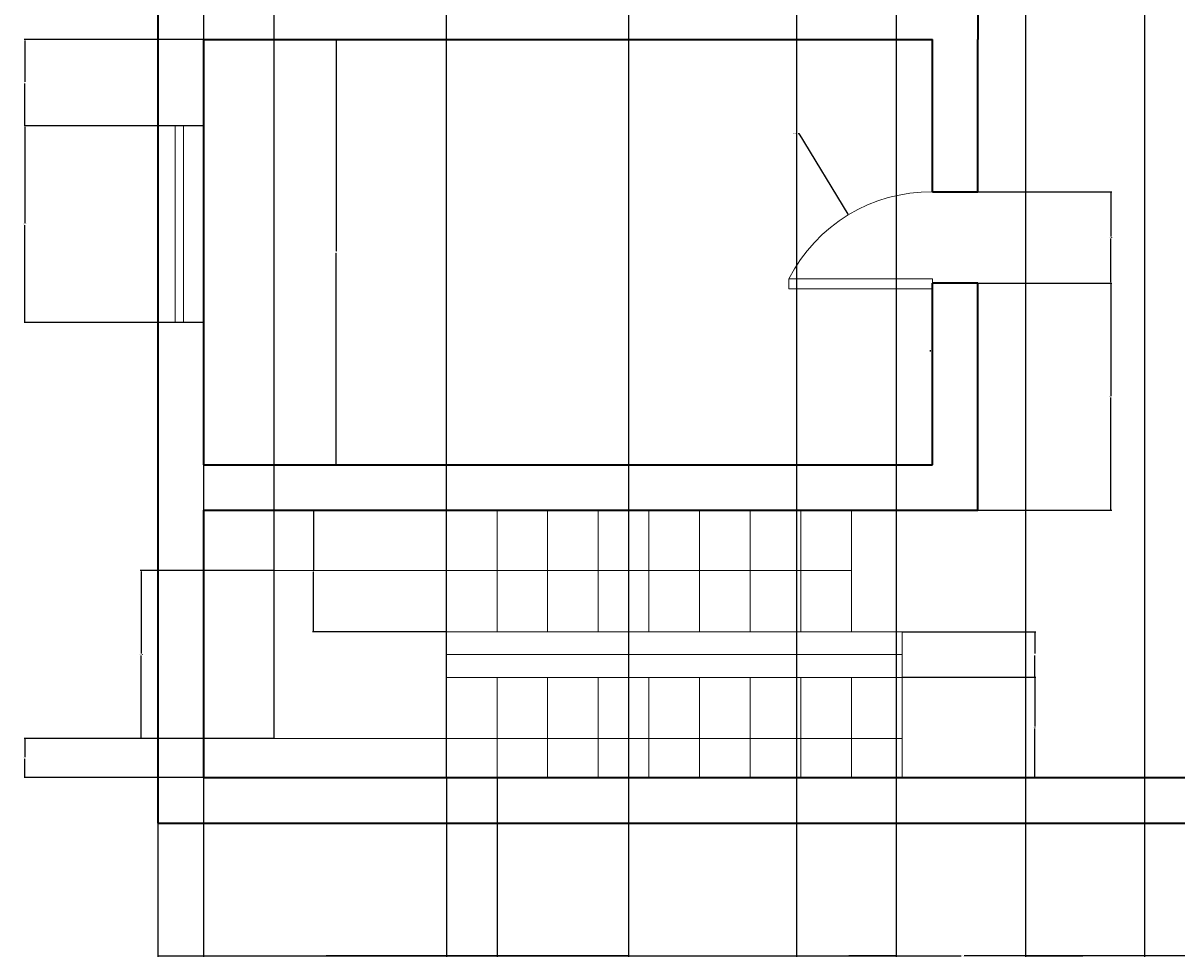
# Model space of a CAD drawing. Units: inches. Extents: x -20 to 351, y -512 to 63.
# Tile 1 of 5: x -20 to 208, y -512 to -328. Entities that reach past the tile are written whole.
import ezdxf

# ---------------------------------------------------------------- set-up
doc = ezdxf.new("R2010")
doc.units = ezdxf.units.IN
doc.header["$MEASUREMENT"] = 0
for name, color, linetype, lineweight in [('A-ANNO-DIMS', 2, 'Continuous', 18), ('A-DOOR', 3, 'Continuous', 18), ('A-FLOR-STRS', 7, 'Continuous', 18), ('A-GLAZ', 4, 'Continuous', 18), ('A-WALL', 7, 'Continuous', 35)]:
    doc.layers.add(name, color=color, linetype=linetype, lineweight=lineweight)
doc.styles.get("Standard").update_dxf_attribs({"font": 'arial.ttf'})
doc.dimstyles.get("Standard").update_dxf_attribs({"dimtxt": 0.18, "dimasz": 0.18, "dimexe": 0.18, "dimexo": 0.0625, "dimgap": 0.09, "dimtad": 0, "dimtih": 1, "dimtoh": 1, "dimdec": 4, "dimzin": 0, "dimdsep": 46, "dimtxsty": 'Standard', "dimcen": 0.09, "dimadec": 0, "dimazin": 0, "dimtfac": 1, "dimtdec": 4, "dimtofl": 0, "dimtmove": 0, "dimatfit": 3, "dimfxl": 1, "dimtolj": 1, "dimtzin": 0, "dimarcsym": 0})

# ---------------------------------------------------------------- blocks, each defined once
blk = doc.blocks.new('*D9')
at = {"layer": 'A-ANNO-DIMS', "color": 0, "lineweight": -2, "transparency": 16777216}
for p, q in [((324.28, -315.88), (324.28, -512.19)), ((6.28, -485.83), (6.28, -512.19)), ((6.46, -512.01), (165, -512.01)), ((324.1, -512.01), (165.57, -512.01))]:
    blk.add_line(p, q, dxfattribs=at)
at = {"layer": 'A-ANNO-DIMS', "color": 0, "transparency": 16777216}
for points in [[(6.46, -511.98), (6.46, -512.04), (6.28, -512.01)], [(324.1, -511.98), (324.1, -512.04), (324.28, -512.01)]]:
    blk.add_solid(points, dxfattribs=at)
at = {"layer": 'Defpoints', "color": 0, "transparency": 16777216}
for p in [(324.28, -315.82), (6.28, -485.76), (324.28, -512.01)]:
    blk.add_point(p, dxfattribs=at)
at = {"layer": 'A-ANNO-DIMS', "color": 0, "transparency": 16777216, "insert": (165.28, -512.01), "char_height": 0.18, "attachment_point": 5}
blk.add_mtext('\\A1;318', dxfattribs=at)
blk = doc.blocks.new('*D20')
at = {"layer": 'A-ANNO-DIMS', "color": 0, "lineweight": -2, "transparency": 16777216}
for p, q in [((15.22, -330.96), (-20.15, -330.96)), ((-19.97, -331.14), (-19.97, -339.31)), ((-19.97, -347.84), (-19.97, -339.67)), ((15.22, -348.02), (-20.15, -348.02))]:
    blk.add_line(p, q, dxfattribs=at)
at = {"layer": 'A-ANNO-DIMS', "color": 0, "transparency": 16777216}
for points in [[(-20, -331.14), (-19.94, -331.14), (-19.97, -330.96)], [(-20, -347.84), (-19.94, -347.84), (-19.97, -348.02)]]:
    blk.add_solid(points, dxfattribs=at)
at = {"layer": 'Defpoints', "color": 0, "transparency": 16777216}
for p in [(15.28, -330.96), (-19.97, -348.02), (15.28, -348.02)]:
    blk.add_point(p, dxfattribs=at)
at = {"layer": 'A-ANNO-DIMS', "color": 0, "transparency": 16777216, "insert": (-19.97, -339.49), "char_height": 0.18, "attachment_point": 5}
blk.add_mtext('\\A1;17.053', dxfattribs=at)
blk = doc.blocks.new('*D21')
at = {"layer": 'A-ANNO-DIMS', "color": 0, "lineweight": -2, "transparency": 16777216}
for p, q in [((15.22, -348.02), (-20.15, -348.02)), ((-19.97, -348.2), (-19.97, -367.28)), ((-19.97, -386.72), (-19.97, -367.64)), ((15.22, -386.9), (-20.15, -386.9))]:
    blk.add_line(p, q, dxfattribs=at)
at = {"layer": 'A-ANNO-DIMS', "color": 0, "transparency": 16777216}
for points in [[(-20, -348.2), (-19.94, -348.2), (-19.97, -348.02)], [(-20, -386.72), (-19.94, -386.72), (-19.97, -386.9)]]:
    blk.add_solid(points, dxfattribs=at)
at = {"layer": 'Defpoints', "color": 0, "transparency": 16777216}
for p in [(15.28, -348.02), (-19.97, -386.9), (15.28, -386.9)]:
    blk.add_point(p, dxfattribs=at)
at = {"layer": 'A-ANNO-DIMS', "color": 0, "transparency": 16777216, "insert": (-19.97, -367.46), "char_height": 0.18, "attachment_point": 5}
blk.add_mtext('\\A1;38.88', dxfattribs=at)
blk = doc.blocks.new('*D22')
at = {"layer": 'A-ANNO-DIMS', "color": 0, "lineweight": -2, "transparency": 16777216}
for p, q in [((15.35, -330.96), (41.71, -330.96)), ((41.53, -331.14), (41.53, -372.78)), ((41.53, -414.78), (41.53, -373.15)), ((15.35, -414.96), (41.71, -414.96))]:
    blk.add_line(p, q, dxfattribs=at)
at = {"layer": 'A-ANNO-DIMS', "color": 0, "transparency": 16777216}
for points in [[(41.5, -331.14), (41.56, -331.14), (41.53, -330.96)], [(41.5, -414.78), (41.56, -414.78), (41.53, -414.96)]]:
    blk.add_solid(points, dxfattribs=at)
at = {"layer": 'Defpoints', "color": 0, "transparency": 16777216}
for p in [(15.28, -330.96), (15.28, -414.96), (41.53, -414.96)]:
    blk.add_point(p, dxfattribs=at)
at = {"layer": 'A-ANNO-DIMS', "color": 0, "transparency": 16777216, "insert": (41.53, -372.96), "char_height": 0.18, "attachment_point": 5}
blk.add_mtext('\\A1;84', dxfattribs=at)
blk = doc.blocks.new('*D35')
at = {"layer": 'A-ANNO-DIMS', "color": 0, "lineweight": -2, "transparency": 16777216}
for p, q in [((15.28, -181.03), (15.28, -512.19)), ((99.28, -181.03), (99.28, -512.19)), ((15.46, -512.01), (57.07, -512.01)), ((99.1, -512.01), (57.5, -512.01))]:
    blk.add_line(p, q, dxfattribs=at)
at = {"layer": 'A-ANNO-DIMS', "color": 0, "transparency": 16777216}
for points in [[(15.46, -511.98), (15.46, -512.04), (15.28, -512.01)], [(99.1, -511.98), (99.1, -512.04), (99.28, -512.01)]]:
    blk.add_solid(points, dxfattribs=at)
at = {"layer": 'Defpoints', "color": 0, "transparency": 16777216}
for p in [(15.28, -180.96), (99.28, -180.96), (99.28, -512.01)]:
    blk.add_point(p, dxfattribs=at)
at = {"layer": 'A-ANNO-DIMS', "color": 0, "transparency": 16777216, "insert": (57.28, -512.01), "char_height": 0.18, "attachment_point": 5}
blk.add_mtext('\\A1;84', dxfattribs=at)
blk = doc.blocks.new('*D40')
at = {"layer": 'A-ANNO-DIMS', "color": 0, "lineweight": -2, "transparency": 16777216}
for p, q in [((132.43, -125.83), (132.43, -512.19)), ((152.16, -125.83), (152.16, -512.19)), ((132.61, -512.01), (141.84, -512.01)), ((151.98, -512.01), (142.75, -512.01))]:
    blk.add_line(p, q, dxfattribs=at)
at = {"layer": 'A-ANNO-DIMS', "color": 0, "transparency": 16777216}
for points in [[(132.61, -511.98), (132.61, -512.04), (132.43, -512.01)], [(151.98, -511.98), (151.98, -512.04), (152.16, -512.01)]]:
    blk.add_solid(points, dxfattribs=at)
at = {"layer": 'Defpoints', "color": 0, "transparency": 16777216}
for p in [(132.43, -125.76), (152.16, -125.76), (132.43, -512.01)]:
    blk.add_point(p, dxfattribs=at)
at = {"layer": 'A-ANNO-DIMS', "color": 0, "transparency": 16777216, "insert": (142.3, -512.01), "char_height": 0.18, "attachment_point": 5}
blk.add_mtext('\\A1;19.727', dxfattribs=at)
blk = doc.blocks.new('*D42')
at = {"layer": 'A-ANNO-DIMS', "color": 0, "lineweight": -2, "transparency": 16777216}
for p, q in [((177.69, -125.83), (177.69, -512.19)), ((201.2, -125.83), (201.2, -512.19)), ((177.87, -512.01), (188.98, -512.01)), ((201.02, -512.01), (189.91, -512.01))]:
    blk.add_line(p, q, dxfattribs=at)
at = {"layer": 'A-ANNO-DIMS', "color": 0, "transparency": 16777216}
for points in [[(177.87, -511.98), (177.87, -512.04), (177.69, -512.01)], [(201.02, -511.98), (201.02, -512.04), (201.2, -512.01)]]:
    blk.add_solid(points, dxfattribs=at)
at = {"layer": 'Defpoints', "color": 0, "transparency": 16777216}
for p in [(177.69, -125.76), (201.2, -125.76), (201.2, -512.01)]:
    blk.add_point(p, dxfattribs=at)
at = {"layer": 'A-ANNO-DIMS', "color": 0, "transparency": 16777216, "insert": (189.45, -512.01), "char_height": 0.18, "attachment_point": 5}
blk.add_mtext('\\A1;23.516', dxfattribs=at)
blk = doc.blocks.new('*D49')
at = {"layer": 'A-ANNO-DIMS', "color": 0, "lineweight": -2, "transparency": 16777216}
for p, q in [((168.35, -361.09), (194.71, -361.09)), ((194.53, -361.27), (194.53, -369.9)), ((194.53, -378.89), (194.53, -370.26)), ((168.35, -379.07), (194.71, -379.07))]:
    blk.add_line(p, q, dxfattribs=at)
at = {"layer": 'A-ANNO-DIMS', "color": 0, "transparency": 16777216}
for points in [[(194.5, -361.27), (194.56, -361.27), (194.53, -361.09)], [(194.5, -378.89), (194.56, -378.89), (194.53, -379.07)]]:
    blk.add_solid(points, dxfattribs=at)
at = {"layer": 'Defpoints', "color": 0, "transparency": 16777216}
for p in [(168.28, -361.09), (168.28, -379.07), (194.53, -379.07)]:
    blk.add_point(p, dxfattribs=at)
at = {"layer": 'A-ANNO-DIMS', "color": 0, "transparency": 16777216, "insert": (194.53, -370.08), "char_height": 0.18, "attachment_point": 5}
blk.add_mtext('\\A1;17.98', dxfattribs=at)
blk = doc.blocks.new('*D50')
at = {"layer": 'A-ANNO-DIMS', "color": 0, "lineweight": -2, "transparency": 16777216}
for p, q in [((168.35, -379.07), (194.71, -379.07)), ((194.53, -379.25), (194.53, -401.33)), ((194.53, -423.78), (194.53, -401.7)), ((168.35, -423.96), (194.71, -423.96))]:
    blk.add_line(p, q, dxfattribs=at)
at = {"layer": 'A-ANNO-DIMS', "color": 0, "transparency": 16777216}
for points in [[(194.5, -379.25), (194.56, -379.25), (194.53, -379.07)], [(194.5, -423.78), (194.56, -423.78), (194.53, -423.96)]]:
    blk.add_solid(points, dxfattribs=at)
at = {"layer": 'Defpoints', "color": 0, "transparency": 16777216}
for p in [(168.28, -379.07), (168.28, -423.96), (194.53, -423.96)]:
    blk.add_point(p, dxfattribs=at)
at = {"layer": 'A-ANNO-DIMS', "color": 0, "transparency": 16777216, "insert": (194.53, -401.52), "char_height": 0.18, "attachment_point": 5}
blk.add_mtext('\\A1;44.9', dxfattribs=at)
blk = doc.blocks.new('*D51')
at = {"layer": 'A-ANNO-DIMS', "color": 0, "lineweight": -2, "transparency": 16777216}
for p, q in [((29.23, -468.97), (29.23, 62.67)), ((29.41, 62.49), (45.86, 62.49)), ((63.1, 62.49), (46.65, 62.49)), ((63.28, -476.7), (63.28, 62.67))]:
    blk.add_line(p, q, dxfattribs=at)
at = {"layer": 'A-ANNO-DIMS', "color": 0, "transparency": 16777216}
for points in [[(29.41, 62.52), (29.41, 62.46), (29.23, 62.49)], [(63.1, 62.52), (63.1, 62.46), (63.28, 62.49)]]:
    blk.add_solid(points, dxfattribs=at)
at = {"layer": 'Defpoints', "color": 0, "transparency": 16777216}
for p in [(63.28, 62.49), (29.23, -469.03), (63.28, -476.76)]:
    blk.add_point(p, dxfattribs=at)
at = {"layer": 'A-ANNO-DIMS', "color": 0, "transparency": 16777216, "insert": (46.26, 62.49), "char_height": 0.18, "attachment_point": 5}
blk.add_mtext('\\A1;34.06', dxfattribs=at)
blk = doc.blocks.new('*D52')
at = {"layer": 'A-ANNO-DIMS', "color": 0, "lineweight": -2, "transparency": 16777216}
for p, q in [((63.28, -476.83), (63.28, -512.19)), ((73.28, -476.83), (73.28, -512.19)), ((63.46, -512.01), (68.07, -512.01)), ((73.1, -512.01), (68.49, -512.01))]:
    blk.add_line(p, q, dxfattribs=at)
at = {"layer": 'A-ANNO-DIMS', "color": 0, "transparency": 16777216}
for points in [[(63.46, -511.98), (63.46, -512.04), (63.28, -512.01)], [(73.1, -511.98), (73.1, -512.04), (73.28, -512.01)]]:
    blk.add_solid(points, dxfattribs=at)
at = {"layer": 'Defpoints', "color": 0, "transparency": 16777216}
for p in [(63.28, -476.76), (73.28, -476.76), (73.28, -512.01)]:
    blk.add_point(p, dxfattribs=at)
at = {"layer": 'A-ANNO-DIMS', "color": 0, "transparency": 16777216, "insert": (68.28, -512.01), "char_height": 0.18, "attachment_point": 5}
blk.add_mtext('\\A1;10', dxfattribs=at)
blk = doc.blocks.new('*D53')
at = {"layer": 'A-ANNO-DIMS', "color": 0, "lineweight": -2, "transparency": 16777216}
for p, q in [((63.22, -423.96), (36.85, -423.96)), ((37.03, -424.14), (37.03, -435.78)), ((37.03, -447.78), (37.03, -436.14)), ((63.22, -447.96), (36.85, -447.96))]:
    blk.add_line(p, q, dxfattribs=at)
at = {"layer": 'A-ANNO-DIMS', "color": 0, "transparency": 16777216}
for points in [[(37, -424.14), (37.06, -424.14), (37.03, -423.96)], [(37, -447.78), (37.06, -447.78), (37.03, -447.96)]]:
    blk.add_solid(points, dxfattribs=at)
at = {"layer": 'Defpoints', "color": 0, "transparency": 16777216}
for p in [(37.03, -423.96), (63.28, -423.96), (63.28, -447.96)]:
    blk.add_point(p, dxfattribs=at)
at = {"layer": 'A-ANNO-DIMS', "color": 0, "transparency": 16777216, "insert": (37.03, -435.96), "char_height": 0.18, "attachment_point": 5}
blk.add_mtext('\\A1;24', dxfattribs=at)
blk = doc.blocks.new('*D54')
at = {"layer": 'A-ANNO-DIMS', "color": 0, "lineweight": -2, "transparency": 16777216}
for p, q in [((153.35, -456.96), (179.71, -456.96)), ((179.53, -457.14), (179.53, -466.68)), ((179.53, -476.58), (179.53, -467.05)), ((153.35, -476.76), (179.71, -476.76))]:
    blk.add_line(p, q, dxfattribs=at)
at = {"layer": 'A-ANNO-DIMS', "color": 0, "transparency": 16777216}
for points in [[(179.5, -457.14), (179.56, -457.14), (179.53, -456.96)], [(179.5, -476.58), (179.56, -476.58), (179.53, -476.76)]]:
    blk.add_solid(points, dxfattribs=at)
at = {"layer": 'Defpoints', "color": 0, "transparency": 16777216}
for p in [(153.28, -456.96), (153.28, -476.76), (179.53, -476.76)]:
    blk.add_point(p, dxfattribs=at)
at = {"layer": 'A-ANNO-DIMS', "color": 0, "transparency": 16777216, "insert": (179.53, -466.86), "char_height": 0.18, "attachment_point": 5}
blk.add_mtext('\\A1;19.8', dxfattribs=at)
blk = doc.blocks.new('*D55')
at = {"layer": 'A-ANNO-DIMS', "color": 0, "lineweight": -2, "transparency": 16777216}
for p, q in [((153.35, -447.96), (179.71, -447.96)), ((179.53, -448.14), (179.53, -452.28)), ((179.53, -456.78), (179.53, -452.65)), ((153.35, -456.96), (179.71, -456.96))]:
    blk.add_line(p, q, dxfattribs=at)
at = {"layer": 'A-ANNO-DIMS', "color": 0, "transparency": 16777216}
for points in [[(179.5, -448.14), (179.56, -448.14), (179.53, -447.96)], [(179.5, -456.78), (179.56, -456.78), (179.53, -456.96)]]:
    blk.add_solid(points, dxfattribs=at)
at = {"layer": 'Defpoints', "color": 0, "transparency": 16777216}
for p in [(153.28, -447.96), (153.28, -456.96), (179.53, -456.96)]:
    blk.add_point(p, dxfattribs=at)
at = {"layer": 'A-ANNO-DIMS', "color": 0, "transparency": 16777216, "insert": (179.53, -452.46), "char_height": 0.18, "attachment_point": 5}
blk.add_mtext('\\A1;9', dxfattribs=at)
blk = doc.blocks.new('*D56')
at = {"layer": 'A-ANNO-DIMS', "color": 0, "lineweight": -2, "transparency": 16777216}
for p, q in [((15.28, -476.83), (15.28, -512.19)), ((63.28, -476.83), (63.28, -512.19)), ((15.46, -512.01), (39.06, -512.01)), ((63.1, -512.01), (39.51, -512.01))]:
    blk.add_line(p, q, dxfattribs=at)
at = {"layer": 'A-ANNO-DIMS', "color": 0, "transparency": 16777216}
for points in [[(15.46, -511.98), (15.46, -512.04), (15.28, -512.01)], [(63.1, -511.98), (63.1, -512.04), (63.28, -512.01)]]:
    blk.add_solid(points, dxfattribs=at)
at = {"layer": 'Defpoints', "color": 0, "transparency": 16777216}
for p in [(15.28, -476.76), (63.28, -476.76), (63.28, -512.01)]:
    blk.add_point(p, dxfattribs=at)
at = {"layer": 'A-ANNO-DIMS', "color": 0, "transparency": 16777216, "insert": (39.28, -512.01), "char_height": 0.18, "attachment_point": 5}
blk.add_mtext('\\A1;48', dxfattribs=at)
blk = doc.blocks.new('*D74')
at = {"layer": 'A-ANNO-DIMS', "color": 0, "lineweight": -2, "transparency": 16777216}
for p, q in [((29.16, -435.87), (2.8, -435.87)), ((2.98, -436.05), (2.98, -452.27)), ((2.98, -468.85), (2.98, -452.63)), ((29.16, -469.03), (2.8, -469.03))]:
    blk.add_line(p, q, dxfattribs=at)
at = {"layer": 'A-ANNO-DIMS', "color": 0, "transparency": 16777216}
for points in [[(2.95, -436.05), (3.01, -436.05), (2.98, -435.87)], [(2.95, -468.85), (3.01, -468.85), (2.98, -469.03)]]:
    blk.add_solid(points, dxfattribs=at)
at = {"layer": 'Defpoints', "color": 0, "transparency": 16777216}
for p in [(2.98, -435.87), (29.23, -435.87), (29.23, -469.03)]:
    blk.add_point(p, dxfattribs=at)
at = {"layer": 'A-ANNO-DIMS', "color": 0, "transparency": 16777216, "insert": (2.98, -452.45), "char_height": 0.18, "attachment_point": 5}
blk.add_mtext('\\A1;33.156', dxfattribs=at)
blk = doc.blocks.new('*D75')
at = {"layer": 'A-ANNO-DIMS', "color": 0, "lineweight": -2, "transparency": 16777216}
for p, q in [((29.16, -469.03), (-20.15, -469.03)), ((-19.97, -469.21), (-19.97, -472.71)), ((-19.97, -476.58), (-19.97, -473.08)), ((15.22, -476.76), (-20.15, -476.76))]:
    blk.add_line(p, q, dxfattribs=at)
at = {"layer": 'A-ANNO-DIMS', "color": 0, "transparency": 16777216}
for points in [[(-20, -469.21), (-19.94, -469.21), (-19.97, -469.03)], [(-20, -476.58), (-19.94, -476.58), (-19.97, -476.76)]]:
    blk.add_solid(points, dxfattribs=at)
at = {"layer": 'Defpoints', "color": 0, "transparency": 16777216}
for p in [(29.23, -469.03), (-19.97, -476.76), (15.28, -476.76)]:
    blk.add_point(p, dxfattribs=at)
at = {"layer": 'A-ANNO-DIMS', "color": 0, "transparency": 16777216, "insert": (-19.97, -472.9), "char_height": 0.18, "attachment_point": 5}
blk.add_mtext('\\A1;7.735', dxfattribs=at)
blk = doc.blocks.new('*D80')
at = {"layer": 'A-ANNO-DIMS', "color": 0, "lineweight": -2, "transparency": 16777216}
for p, q in [((132.74, -349.52), (132.92, -349.52)), ((132.92, -349.52), (142.57, -365.46)), ((158.81, -392.44), (158.99, -392.44)), ((158.9, -392.53), (158.9, -392.35))]:
    blk.add_line(p, q, dxfattribs=at)
at = {"layer": 'A-ANNO-DIMS', "color": 0, "transparency": 16777216}
blk.add_solid([(142.59, -365.45), (142.54, -365.48), (142.66, -365.62)], dxfattribs=at)
at = {"layer": 'Defpoints', "color": 0, "transparency": 16777216}
for p in [(142.66, -365.62), (158.9, -392.44)]:
    blk.add_point(p, dxfattribs=at)
at = {"layer": 'A-ANNO-DIMS', "color": 0, "transparency": 16777216, "insert": (132.26, -349.52), "char_height": 0.18, "attachment_point": 5}
blk.add_mtext('\\A1;R31.36', dxfattribs=at)

msp = doc.modelspace()

# ---------------------------------------------------------------- linework, layer by layer
at = {"layer": 'A-DOOR'}
for p, q in [((130.9395, -378.2457), (159.2844, -378.2457)), ((130.9395, -380.2094), (130.9395, -378.2457)), ((159.2844, -378.2457), (159.2844, -380.2094)), ((130.9395, -380.2094), (159.2844, -380.2094)), ((158.4428, -380.2094), (158.4428, -380.2121))]:
    msp.add_line(p, q, dxfattribs=at)
msp.add_arc((158.9005, -392.4444), 31.3596, 89.298544, 153.078365, dxfattribs=at)
at = {"layer": 'A-FLOR-STRS'}
for p, q in [((15.2844, -423.9646), (63.2844, -423.9646)), ((63.2844, -423.9646), (63.2844, -476.7646)), ((63.2844, -423.9646), (68.2844, -423.9646)), ((63.2844, -423.9646), (73.2844, -423.9646)), ((63.2844, -423.9646), (63.2844, -447.9646)), ((73.2844, -423.9646), (73.2844, -447.9646)), ((83.2844, -423.9646), (93.2844, -423.9646)), ((83.2844, -447.9646), (83.2844, -423.9646)), ((93.2844, -423.9646), (93.2844, -447.9646)), ((103.2844, -423.9646), (113.2844, -423.9646)), ((103.2844, -447.9646), (103.2844, -423.9646)), ((113.2844, -423.9646), (113.2844, -447.9646)), ((123.2844, -423.9646), (133.2844, -423.9646)), ((123.2844, -447.9646), (123.2844, -423.9646)), ((133.2844, -423.9646), (133.2844, -447.9646)), ((143.2844, -423.9646), (153.2844, -423.9646)), ((143.2844, -447.9646), (143.2844, -423.9646)), ((143.2844, -435.8733), (29.2263, -435.8733)), ((29.2263, -435.8733), (29.2263, -469.0292)), ((63.2844, -447.9646), (153.2844, -447.9646)), ((153.2844, -447.9646), (153.2844, -476.7646)), ((63.2844, -452.4359), (153.2844, -452.4359)), ((63.2844, -456.9646), (153.2844, -456.9646)), ((73.2844, -456.9646), (73.2844, -476.7646)), ((83.2844, -476.7646), (83.2844, -456.9646)), ((93.2844, -456.9646), (93.2844, -476.7646)), ((103.2844, -476.7646), (103.2844, -456.9646)), ((113.2844, -456.9646), (113.2844, -476.7646)), ((123.2844, -476.7646), (123.2844, -456.9646)), ((133.2844, -456.9646), (133.2844, -476.7646)), ((143.2844, -476.7646), (143.2844, -456.9646)), ((29.2263, -469.0292), (153.2844, -469.0292)), ((73.2844, -476.7646), (83.2844, -476.7646)), ((93.2844, -476.7646), (103.2844, -476.7646)), ((113.2844, -476.7646), (123.2844, -476.7646)), ((133.2844, -476.7646), (143.2844, -476.7646)), ((153.2844, -476.7646), (163.2844, -476.7646))]:
    msp.add_line(p, q, dxfattribs=at)
at = {"layer": 'A-GLAZ'}
for p, q in [((9.7175, -348.0179), (9.7175, -386.9004)), ((11.3534, -348.0179), (11.3534, -386.9004))]:
    msp.add_line(p, q, dxfattribs=at)
msp.add_lwpolyline([(6.2844, -348.0179), (15.2844, -348.0179), (15.2844, -386.9004), (6.2844, -386.9004)], close=True, dxfattribs=at)
at = {"layer": 'A-WALL'}
for p, q in [((6.2844, 36.2354), (6.2844, -476.7646)), ((168.2844, -298.9325), (168.2844, -330.9646)), ((15.2844, -330.9646), (159.2844, -330.9646)), ((15.2844, -330.9646), (15.2844, -414.9646)), ((15.2844, -330.9646), (15.2844, -414.9646)), ((159.2844, -361.0872), (159.2844, -330.9646)), ((168.2844, -361.0872), (168.2844, -330.9646)), ((159.2844, -361.0872), (168.2844, -361.0872)), ((159.2844, -414.9646), (159.2844, -379.0683)), ((168.2844, -379.0683), (159.2844, -379.0683)), ((168.2844, -423.9646), (168.2844, -379.0683)), ((15.2844, -414.9646), (159.2844, -414.9646)), ((15.2844, -423.9646), (168.2844, -423.9646)), ((15.2844, -423.9646), (15.2844, -476.7646)), ((6.2844, -476.7646), (6.2844, -485.7646)), ((15.2844, -476.7646), (228.604, -476.7646)), ((6.2844, -485.7646), (228.604, -485.7646))]:
    msp.add_line(p, q, dxfattribs=at)

# ---------------------------------------------------------------- dimensions: what is measured, and where the dimension line sits
at = {"layer": 'A-ANNO-DIMS'}
for base, p1, p2, override, picture, middle in [((63.2844, 62.4854), (29.2263, -469.0292), (63.2844, -476.7646), {"dimdec": 2, "dimlfac": 1, "dimrnd": 0, "dimzin": 0, "dimdsep": 46, "dimlunit": 2}, '*D51', (46.2554, 62.4854)), ((132.4341, -512.0146), (152.1609, -125.7646), (132.4341, -125.7646), {"dimdec": 3, "dimlfac": 1, "dimrnd": 0, "dimzin": 0, "dimdsep": 46, "dimlunit": 2}, '*D40', (142.2975, -512.0146)), ((201.2048, -512.0146), (177.6888, -125.7646), (201.2048, -125.7646), {"dimdec": 3, "dimlfac": 1, "dimrnd": 0, "dimzin": 0, "dimdsep": 46, "dimlunit": 2}, '*D42', (189.4468, -512.0146)), ((99.2844, -512.0146), (15.2844, -180.9646), (99.2844, -180.9646), {"dimdec": 0, "dimlfac": 1, "dimrnd": 0, "dimzin": 0, "dimdsep": 46, "dimlunit": 2}, '*D35', (57.2844, -512.0146)), ((324.2844, -512.0146), (6.2844, -485.7646), (324.2844, -315.8223), {"dimdec": 0, "dimlfac": 1, "dimrnd": 0, "dimzin": 0, "dimdsep": 46, "dimlunit": 2}, '*D9', (165.2844, -512.0146)), ((63.2844, -512.0146), (15.2844, -476.7646), (63.2844, -476.7646), {"dimdec": 0, "dimlfac": 1, "dimrnd": 0, "dimzin": 0, "dimdsep": 46, "dimlunit": 2}, '*D56', (39.2844, -512.0146)), ((73.2844, -512.0146), (63.2844, -476.7646), (73.2844, -476.7646), {"dimdec": 0, "dimlfac": 1, "dimrnd": 0, "dimzin": 0, "dimdsep": 46, "dimlunit": 2}, '*D52', (68.2844, -512.0146))]:
    dim = msp.add_linear_dim(base=base, p1=p1, p2=p2, dimstyle='Standard', override=override, dxfattribs=at)
    dim.commit()
    dim.dimension.update_dxf_attribs({"geometry": picture, "text_midpoint": middle})
for base, p1, p2, angle, override, picture, middle in [((-19.9656, -348.0179), (15.2844, -330.9646), (15.2844, -348.0179), 90, {"dimdec": 3, "dimlfac": 1, "dimrnd": 0, "dimzin": 0, "dimdsep": 46, "dimlunit": 2}, '*D20', (-19.9656, -339.4913)), ((41.5345, -414.9646), (15.2844, -330.9646), (15.2844, -414.9646), 270, {"dimdec": 0, "dimlfac": 1, "dimrnd": 0, "dimzin": 0, "dimdsep": 46, "dimlunit": 2}, '*D22', (41.5344, -372.9646)), ((-19.9656, -386.9004), (15.2844, -348.0179), (15.2844, -386.9004), 90, {"dimdec": 2, "dimlfac": 1, "dimrnd": 0, "dimzin": 0, "dimdsep": 46, "dimlunit": 2}, '*D21', (-19.9656, -367.4591)), ((194.5345, -379.0683), (168.2844, -361.0872), (168.2844, -379.0683), 270, {"dimdec": 2, "dimlfac": 1, "dimrnd": 0, "dimzin": 0, "dimdsep": 46, "dimlunit": 2}, '*D49', (194.5344, -370.0777)), ((194.5345, -423.9646), (168.2844, -379.0683), (168.2844, -423.9646), 270, {"dimdec": 1, "dimlfac": 1, "dimrnd": 0, "dimzin": 0, "dimdsep": 46, "dimlunit": 2}, '*D50', (194.5344, -401.5165)), ((37.0345, -423.9646), (63.2844, -447.9646), (63.2844, -423.9646), 90, {"dimdec": 0, "dimlfac": 1, "dimrnd": 0, "dimzin": 0, "dimdsep": 46, "dimlunit": 2}, '*D53', (37.0344, -435.9646)), ((2.9763, -435.8733), (29.2263, -469.0292), (29.2263, -435.8733), 90, {"dimdec": 3, "dimlfac": 1, "dimrnd": 0, "dimzin": 0, "dimdsep": 46, "dimlunit": 2}, '*D74', (2.9763, -452.4512)), ((179.5345, -456.9646), (153.2844, -447.9646), (153.2844, -456.9646), 270, {"dimdec": 0, "dimlfac": 1, "dimrnd": 0, "dimzin": 0, "dimdsep": 46, "dimlunit": 2}, '*D55', (179.5344, -452.4646)), ((179.5345, -476.7646), (153.2844, -456.9646), (153.2844, -476.7646), 270, {"dimdec": 1, "dimlfac": 1, "dimrnd": 0, "dimzin": 0, "dimdsep": 46, "dimlunit": 2}, '*D54', (179.5344, -466.8646)), ((-19.9656, -476.7646), (29.2263, -469.0292), (15.2844, -476.7646), 90, {"dimdec": 3, "dimlfac": 1, "dimrnd": 0, "dimzin": 0, "dimdsep": 46, "dimlunit": 2}, '*D75', (-19.9656, -472.8969))]:
    dim = msp.add_linear_dim(base=base, p1=p1, p2=p2, angle=angle, dimstyle='Standard', override=override, dxfattribs=at)
    dim.commit()
    dim.dimension.update_dxf_attribs({"geometry": picture, "text_midpoint": middle})
dim = msp.add_radius_dim(center=(158.9005, -392.4444), mpoint=(142.6611, -365.6171), dimstyle='Standard', override={"dimdec": 2, "dimlfac": 1, "dimrnd": 0, "dimzin": 0, "dimdsep": 46, "dimlunit": 2}, dxfattribs=at)
dim.commit()
dim.dimension.update_dxf_attribs({"geometry": '*D80', "text_midpoint": (132.2576, -349.5207), "dimtype": 164})

doc.saveas('drawing.dxf')
